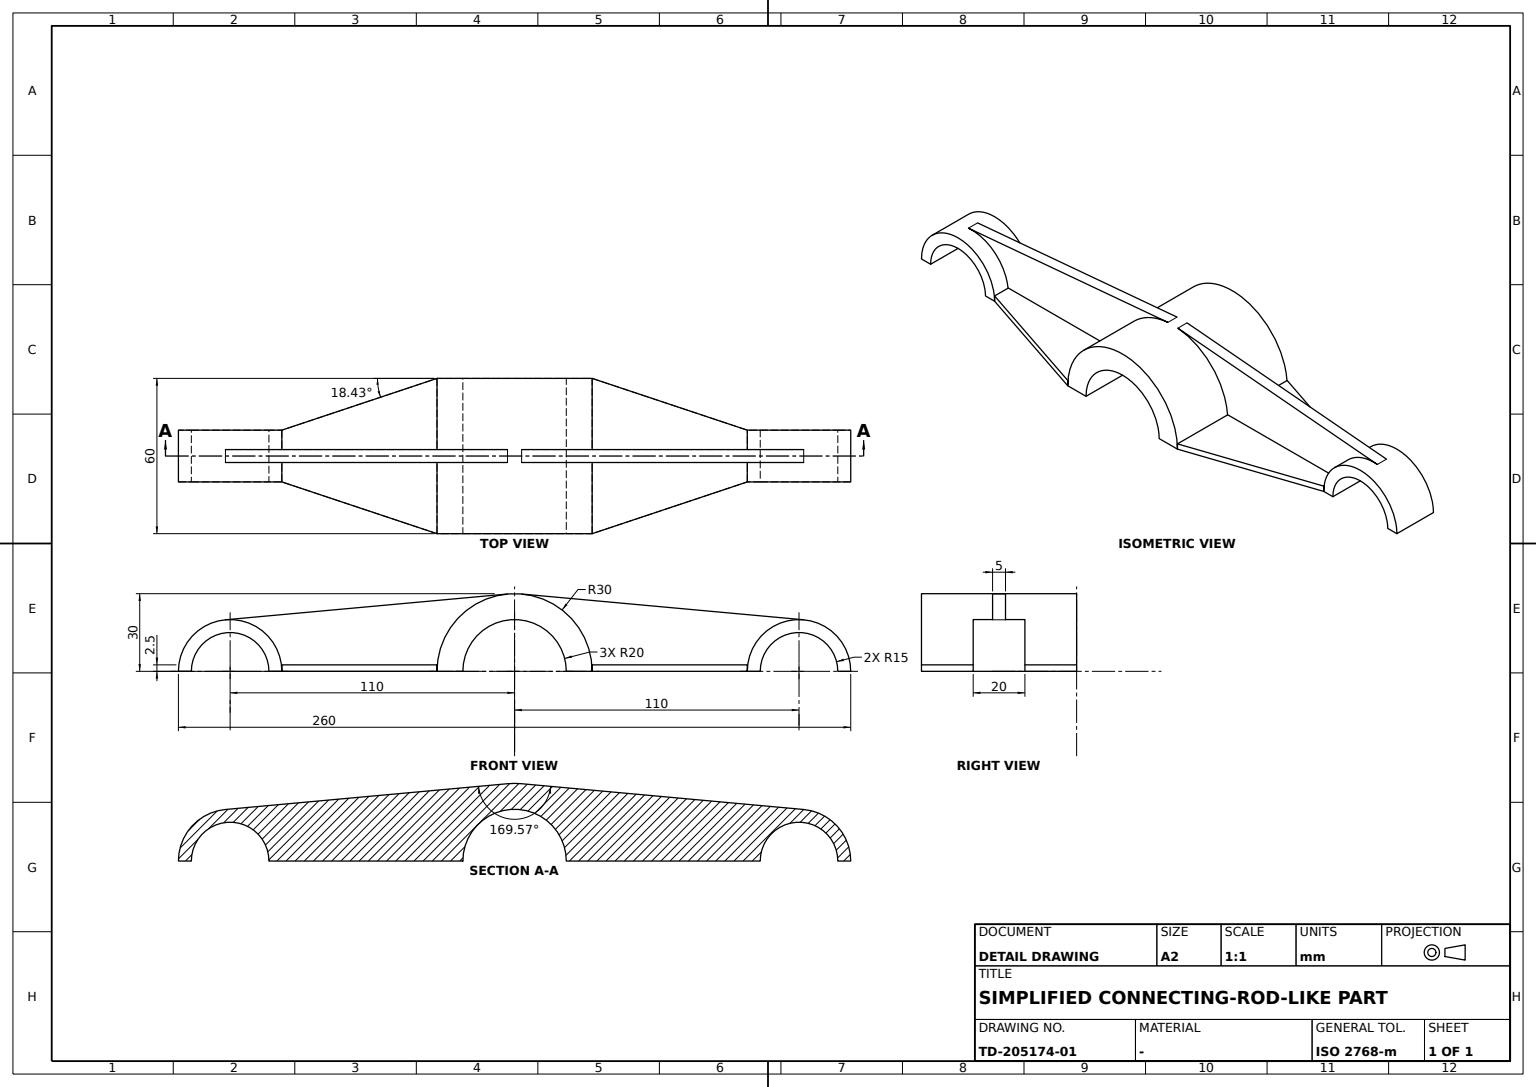
CATIA V5 part; units mm, degrees
sketch "Sketch1" plane through (0, 0, 0) normal (0, 1, 0) x (-1, 0, 0)
  arc A0 (30, 0) -> (-30, 0) centre (0, 0) ccw
  arc A1 (20, 0) -> (-20, 0) centre (0, 0) ccw
  line L0 (-30, 0) -> (-20, 0)
  line L1 (20, 0) -> (30, 0)
  dimension "radius A1" = 20
  dimension "radius A0" = 30
  constraint horizontal L0 x-axis
  constraint horizontal L1 x-axis
  constraint coincidence L0 L1
  constraint coincidence L1 origin
extrude "Pad1" add sketch "Sketch1" along normal mid plane 60
sketch "Sketch2" plane through (0, 0, 0) normal (0, 1, 0) x (-1, 0, 0)
  arc A0 (-90, 0) -> (-130, 0) centre (-110, 0) ccw
  point P0 (-110, 0)
  arc A1 (-95, 0) -> (-125, 0) centre (-110, 0) ccw
  arc A2 (130, 0) -> (90, 0) centre (110, 0) ccw
  point P1 (110, 0)
  arc A3 (125, 0) -> (95, 0) centre (110, 0) ccw
  line L0 (130, 0) -> (125, 0)
  point P2 (-90, 0)
  point P3 (-125, 0)
  line L1 (-125, 0) -> (-130, 0)
  line L2 (-90, 0) -> (-95, 0)
  point P4 (95, 0)
  line L3 (95, 0) -> (90, 0)
  dimension "radius A3" = 15
  dimension "radius A2" = 20
  dimension "radius A0" = 20
  dimension "radius A1" = 15
  dimension "distance P0 P1" = 220
  dimension "distance P0 origin" = 110
  constraint coincidence P0 x-axis
  constraint coincidence P1 x-axis
  constraint coincidence L0 P2
  constraint coincidence L0 P3
  constraint coincidence L0 L1
  constraint coincidence L0 L2
  constraint coincidence L0 P4
  constraint coincidence L0 L3
  constraint coincidence origin L3
  constraint horizontal L0 x-axis
  constraint horizontal L1 x-axis
  constraint horizontal L2 x-axis
  constraint horizontal L3 x-axis
extrude "Pad2" add sketch "Sketch2" along normal mid plane 20
sketch "Sketch3" plane through (0, 0, 0) normal (0, 0, -1) x (1, 0, 0)
  line L0 (-90, 10) -> (-90, -10)
  point P0 (-90, -10)
  line L1 (-30, 30) -> (-30, -30)
  line L2 (30, 30) -> (30, -30)
  line L3 (90, 10) -> (90, -10)
  line L4 (-90, 10) -> (-30, 30)
  line L5 (30, 30) -> (90, 10)
  line L6 (30, -30) -> (90, -10)
  line L7 (-30, -30) -> (-90, -10)
  point P1 (-90, -10)
  constraint parallelism L6 L4
  constraint parallelism L7 L5
  constraint coincidence P0 P1
extrude "Pad3" add sketch "Sketch3" against normal blind 2.5
sketch "Sketch4" plane through (0, 0, 0) normal (0, 1, 0) x (-1, 0, 0)
  line L0 (2.7273, 29.8758) -> (111.8182, 19.9172)
  point P0 (2.7273, 29.8758)
  point P1 (111.8182, 19.9172)
  arc A0 (130, 0) -> (90, 0) centre (110, 0) ccw construction
  arc A1 (30, 0) -> (-30, 0) centre (0, 0) ccw construction
  arc A2 (130, 0) -> (90, 0) centre (110, 0) ccw construction
  arc A3 (30, 0) -> (-30, 0) centre (0, 0) ccw construction
  point P2 (-111.8182, 19.9172)
  point P3 (-2.7273, 29.8758)
  line L1 (-2.7273, 29.8758) -> (-111.8182, 19.9172)
  line L2 (-30, 0) -> (-90, 0)
  point P4 (-30, 0)
  point P5 (-90, 0)
  arc A4 (-90, 0) -> (-111.8182, 19.9172) centre (-110, 0) ccw
  point P6 (-90, 0)
  arc A5 (30, 0) -> (2.7273, 29.8758) centre (0, 0) ccw
  arc A6 (-2.7273, 29.8758) -> (-30, 0) centre (0, 0) ccw
  point P7 (30, 0)
  point P8 (-30, 0)
  line L3 (90, 0) -> (30, 0)
  point P9 (90, 0)
  point P10 (30, 0)
  arc A7 (111.8182, 19.9172) -> (90, 0) centre (110, 0) ccw
  point P11 (90, 0)
  constraint coincidence P1 A0
  constraint coincidence P0 A3
  constraint coincidence P4 P8
  constraint coincidence P5 P6
  constraint coincidence P7 P10
  constraint coincidence P9 P11
  constraint tangency L0 A1
  constraint tangency L0 A2
  constraint symmetry P1 P2 y-axis
  constraint symmetry P0 P3 y-axis
  constraint symmetry L0 L1 y-axis
extrude "Pad4" add sketch "Sketch4" along normal mid plane 5
